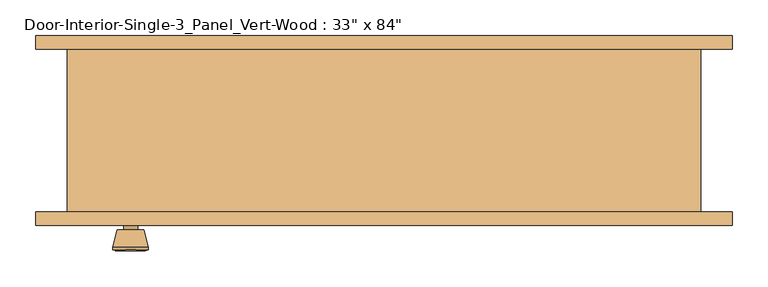
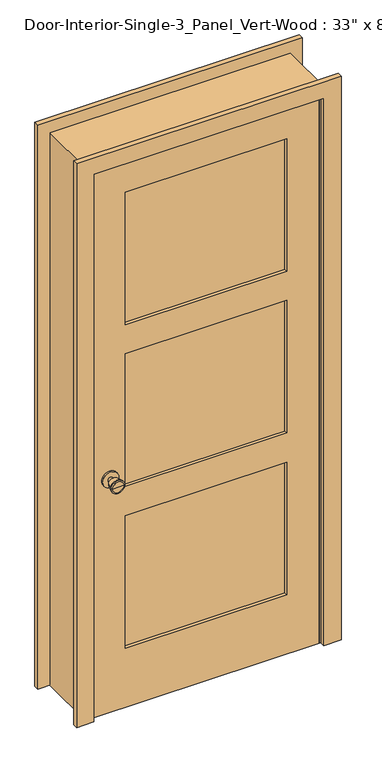
"""IFC4 building model written with IfcOpenShell, lengths in millimetres: door geometry."""

from ifc_helpers import new_model, si_unit, point, frame, frame_2d, origin, place, context, project, spatial, polyline, circle_curve, trimmed, segment, composite_curve, outline, extrude, faceted_brep, source, transform, mapped, element, save
from ifc_brep_helpers import plane_surface, cylinder_surface, revolved_surface, advanced_brep


def door_5abea521(model_context):
    return source(origin(), model_context, "Body", "SolidModel", [
        advanced_brep(
        [(-355.6, -70.2, 914.4), (-365.6, -70.2, 914.4), (-345.6, -70.2, 914.4), (-335.1241324, -21.2, 914.4), (-376.0758676, -21.2, 914.4), (-355.6, -21.2, 914.4), (-330.6, -23.0278681, 914.4), (-380.6, -23.0278681, 914.4), (-330.6, -26.4915463, 914.4), (-380.6, -26.4915463, 914.4), (-336.963764, -51.2, 914.4), (-374.236236, -51.2, 914.4), (-345.6, -51.2, 914.4), (-365.6, -51.2, 914.4)],
        [
            (0, 1),
            (1, 2, circle_curve(frame((-355.6, -70.2, 914.4), z_axis=(0.0, -1.0, 0.0), x_axis=(-1.0, 0.0, 0.0)), 10.0)),
            (2, 0),
            (2, 1, circle_curve(frame((-355.6, -70.2, 914.4), z_axis=(0.0, -1.0, 0.0), x_axis=(-1.0, 0.0, 0.0)), 10.0)),
            (3, 4, circle_curve(frame((-355.6, -21.2, 914.4), z_axis=(0.0, 1.0, 0.0), x_axis=(-1.0, 0.0, 0.0)), 20.4758676)),
            (4, 5),
            (5, 3),
            (4, 3, circle_curve(frame((-355.6, -21.2, 914.4), z_axis=(0.0, 1.0, 0.0), x_axis=(-1.0, 0.0, 0.0)), 20.4758676)),
            (6, 7, circle_curve(frame((-355.6, -23.0278681, 914.4), z_axis=(0.0, 1.0, 0.0), x_axis=(-1.0, 0.0, 0.0)), 25.0)),
            (7, 4),
            (3, 6),
            (7, 6, circle_curve(frame((-355.6, -23.0278681, 914.4), z_axis=(0.0, 1.0, 0.0), x_axis=(-1.0, 0.0, 0.0)), 25.0)),
            (8, 9, circle_curve(frame((-355.6, -26.4915463, 914.4), z_axis=(0.0, 1.0, 0.0), x_axis=(-1.0, 0.0, 0.0)), 25.0)),
            (9, 7),
            (6, 8),
            (9, 8, circle_curve(frame((-355.6, -26.4915463, 914.4), z_axis=(0.0, 1.0, 0.0), x_axis=(-1.0, 0.0, 0.0)), 25.0)),
            (10, 11, circle_curve(frame((-355.6, -51.2, 914.4), z_axis=(0.0, 1.0, 0.0), x_axis=(-1.0, 0.0, 0.0)), 18.636236)),
            (11, 9),
            (8, 10),
            (11, 10, circle_curve(frame((-355.6, -51.2, 914.4), z_axis=(0.0, 1.0, 0.0), x_axis=(-1.0, 0.0, 0.0)), 18.636236)),
            (12, 13, circle_curve(frame((-355.6, -51.2, 914.4), z_axis=(0.0, 1.0, 0.0), x_axis=(-1.0, 0.0, 0.0)), 10.0)),
            (13, 11),
            (10, 12),
            (13, 12, circle_curve(frame((-355.6, -51.2, 914.4), z_axis=(0.0, 1.0, 0.0), x_axis=(-1.0, 0.0, 0.0)), 10.0)),
            (1, 13),
            (12, 2),
        ],
        [
            plane_surface(frame((-355.6, -70.2, 914.4), z_axis=(0.0, -1.0, 0.0), x_axis=(-1.0, 0.0, 0.0))),
            plane_surface(frame((-355.6, -21.2, 914.4), z_axis=(0.0, 1.0, 0.0), x_axis=(-1.0, 0.0, 0.0))),
            revolved_surface(polyline([(-376.0758676, -21.2, 914.4), (-380.6, -23.0278681, 914.4)]), (-355.6, -70.2, 914.4), (0.0, -1.0, 0.0)),
            cylinder_surface(frame((-355.6, -70.2, 914.4), z_axis=(0.0, -1.0, 0.0), x_axis=(-1.0, 0.0, 0.0)), 25.0),
            revolved_surface(polyline([(-380.6, -26.4915463, 914.4), (-374.236236, -51.2, 914.4)]), (-355.6, -70.2, 914.4), (0.0, -1.0, 0.0)),
            plane_surface(frame((-355.6, -51.2, 914.4), z_axis=(0.0, -1.0, 0.0), x_axis=(-1.0, 0.0, 0.0))),
            cylinder_surface(frame((-355.6, -70.2, 914.4), z_axis=(0.0, -1.0, 0.0), x_axis=(-1.0, 0.0, 0.0)), 10.0),
        ],
        [
            (0, [[1, 2, 3]]),
            (0, [[-3, 4, -1]]),
            (1, [[5, 6, 7]]),
            (1, [[8, -7, -6]]),
            (2, [[9, 10, -5, 11]]),
            (2, [[12, -11, -8, -10]]),
            (3, [[13, 14, -9, 15]]),
            (3, [[16, -15, -12, -14]]),
            (4, [[17, 18, -13, 19]]),
            (4, [[20, -19, -16, -18]]),
            (5, [[21, 22, -17, 23]]),
            (5, [[24, -23, -20, -22]]),
            (6, [[-2, 25, -21, 26]]),
            (6, [[-4, -26, -24, -25]]),
        ],
    ),
        extrude(outline(composite_curve([segment(trimmed(circle_curve(frame_2d((914.4, -355.6)), 30.0), [point((914.4, -385.6))], [point((914.4, -325.6))], False, "CARTESIAN"), True, "CONTINUOUS"), segment(trimmed(circle_curve(frame_2d((914.4, -355.6)), 30.0), [point((914.4, -325.6))], [point((914.4, -385.6))], False, "CARTESIAN"), True, "CONTINUOUS")], self_intersect=False)), frame((0.0, -76.2, 0.0), z_axis=(0.0, 1.0, 0.0), x_axis=(0.0, 0.0, 1.0)), (0.0, 0.0, 1.0), 6.0),
        advanced_brep(
        [(-355.6, -117.125, 914.4), (-345.6, -117.125, 914.4), (-365.6, -117.125, 914.4), (-335.1241324, -166.125, 914.4), (-355.6, -166.125, 914.4), (-376.0758676, -166.125, 914.4), (-330.6, -164.2971319, 914.4), (-380.6, -164.2971319, 914.4), (-330.6, -160.8334537, 914.4), (-380.6, -160.8334537, 914.4), (-336.963764, -136.125, 914.4), (-374.236236, -136.125, 914.4), (-345.6, -136.125, 914.4), (-365.6, -136.125, 914.4)],
        [
            (0, 1),
            (1, 2, circle_curve(frame((-355.6, -117.125, 914.4), z_axis=(0.0, 1.0, 0.0), x_axis=(-1.0, 0.0, 0.0)), 10.0)),
            (2, 0),
            (2, 1, circle_curve(frame((-355.6, -117.125, 914.4), z_axis=(0.0, 1.0, 0.0), x_axis=(-1.0, 0.0, 0.0)), 10.0)),
            (3, 4),
            (4, 5),
            (5, 3, circle_curve(frame((-355.6, -166.125, 914.4), z_axis=(0.0, -1.0, 0.0), x_axis=(-1.0, 0.0, 0.0)), 20.4758676)),
            (3, 5, circle_curve(frame((-355.6, -166.125, 914.4), z_axis=(0.0, -1.0, 0.0), x_axis=(-1.0, 0.0, 0.0)), 20.4758676)),
            (6, 3),
            (5, 7),
            (7, 6, circle_curve(frame((-355.6, -164.2971319, 914.4), z_axis=(0.0, -1.0, 0.0), x_axis=(-1.0, 0.0, 0.0)), 25.0)),
            (6, 7, circle_curve(frame((-355.6, -164.2971319, 914.4), z_axis=(0.0, -1.0, 0.0), x_axis=(-1.0, 0.0, 0.0)), 25.0)),
            (8, 6),
            (7, 9),
            (9, 8, circle_curve(frame((-355.6, -160.8334537, 914.4), z_axis=(0.0, -1.0, 0.0), x_axis=(-1.0, 0.0, 0.0)), 25.0)),
            (8, 9, circle_curve(frame((-355.6, -160.8334537, 914.4), z_axis=(0.0, -1.0, 0.0), x_axis=(-1.0, 0.0, 0.0)), 25.0)),
            (10, 8),
            (9, 11),
            (11, 10, circle_curve(frame((-355.6, -136.125, 914.4), z_axis=(0.0, -1.0, 0.0), x_axis=(-1.0, 0.0, 0.0)), 18.636236)),
            (10, 11, circle_curve(frame((-355.6, -136.125, 914.4), z_axis=(0.0, -1.0, 0.0), x_axis=(-1.0, 0.0, 0.0)), 18.636236)),
            (12, 10),
            (11, 13),
            (13, 12, circle_curve(frame((-355.6, -136.125, 914.4), z_axis=(0.0, -1.0, 0.0), x_axis=(-1.0, 0.0, 0.0)), 10.0)),
            (12, 13, circle_curve(frame((-355.6, -136.125, 914.4), z_axis=(0.0, -1.0, 0.0), x_axis=(-1.0, 0.0, 0.0)), 10.0)),
            (1, 12),
            (13, 2),
        ],
        [
            plane_surface(frame((-355.6, -117.125, 914.4), z_axis=(0.0, 1.0, 0.0), x_axis=(-1.0, 0.0, 0.0))),
            plane_surface(frame((-355.6, -166.125, 914.4), z_axis=(0.0, -1.0, 0.0), x_axis=(-1.0, 0.0, 0.0))),
            revolved_surface(polyline([(-376.0758676, -166.125, 914.4), (-380.6, -164.2971319, 914.4)]), (-355.6, -117.125, 914.4), (0.0, 1.0, 0.0)),
            cylinder_surface(frame((-355.6, -117.125, 914.4), z_axis=(0.0, 1.0, 0.0), x_axis=(-1.0, 0.0, 0.0)), 25.0),
            revolved_surface(polyline([(-380.6, -160.8334537, 914.4), (-374.236236, -136.125, 914.4)]), (-355.6, -117.125, 914.4), (0.0, 1.0, 0.0)),
            plane_surface(frame((-355.6, -136.125, 914.4), z_axis=(0.0, 1.0, 0.0), x_axis=(-1.0, 0.0, 0.0))),
            cylinder_surface(frame((-355.6, -117.125, 914.4), z_axis=(0.0, 1.0, 0.0), x_axis=(-1.0, 0.0, 0.0)), 10.0),
        ],
        [
            (0, [[1, 2, 3]]),
            (0, [[-3, 4, -1]]),
            (1, [[5, 6, 7]]),
            (1, [[-6, -5, 8]]),
            (2, [[9, -7, 10, 11]]),
            (2, [[-10, -8, -9, 12]]),
            (3, [[13, -11, 14, 15]]),
            (3, [[-14, -12, -13, 16]]),
            (4, [[17, -15, 18, 19]]),
            (4, [[-18, -16, -17, 20]]),
            (5, [[21, -19, 22, 23]]),
            (5, [[-22, -20, -21, 24]]),
            (6, [[25, -23, 26, -2]]),
            (6, [[-26, -24, -25, -4]]),
        ],
    ),
        extrude(outline(composite_curve([segment(trimmed(circle_curve(frame_2d((914.4, -355.6)), 30.0), [point((914.4, -385.6))], [point((914.4, -325.6))], False, "CARTESIAN"), True, "CONTINUOUS"), segment(trimmed(circle_curve(frame_2d((914.4, -355.6)), 30.0), [point((914.4, -325.6))], [point((914.4, -385.6))], False, "CARTESIAN"), True, "CONTINUOUS")], self_intersect=False)), frame((0.0, -117.125, 0.0), z_axis=(0.0, 1.0, 0.0), x_axis=(0.0, 0.0, 1.0)), (0.0, 0.0, 1.0), 6.0),
        faceted_brep([(444.5, -111.125, 0.0), (419.1, -111.125, 0.0), (419.1, -76.2, 0.0), (406.4, -76.2, 0.0), (406.4, -41.275, 0.0), (419.1, -41.275, 0.0), (419.1, 117.475, 0.0), (444.5, 117.475, 0.0), (444.5, 117.475, 2159.0), (444.5, -111.125, 2159.0), (419.1, 117.475, 2133.6), (-419.1, 117.475, 2133.6), (-419.1, 117.475, 0.0), (-444.5, 117.475, 0.0), (-444.5, 117.475, 2159.0), (419.1, -41.275, 2133.6), (406.4, -41.275, 2120.9), (-406.4, -41.275, 2120.9), (-406.4, -41.275, 0.0), (-419.1, -41.275, 0.0), (-419.1, -41.275, 2133.6), (406.4, -76.2, 2120.9), (419.1, -76.2, 2133.6), (-419.1, -76.2, 2133.6), (-419.1, -76.2, 0.0), (-406.4, -76.2, 0.0), (-406.4, -76.2, 2120.9), (419.1, -111.125, 2133.6), (-444.5, -111.125, 2159.0), (-444.5, -111.125, 0.0), (-419.1, -111.125, 0.0), (-419.1, -111.125, 2133.6)], [[[0, 1, 2, 3, 4, 5, 6, 7]], [[7, 8, 9, 0]], [[6, 10, 11, 12, 13, 14, 8, 7]], [[5, 15, 10, 6]], [[4, 16, 17, 18, 19, 20, 15, 5]], [[3, 21, 16, 4]], [[2, 22, 23, 24, 25, 26, 21, 3]], [[1, 27, 22, 2]], [[0, 9, 28, 29, 30, 31, 27, 1]], [[8, 14, 28, 9]], [[15, 20, 11, 10]], [[21, 26, 17, 16]], [[27, 31, 23, 22]], [[29, 13, 12, 19, 18, 25, 24, 30]], [[14, 13, 29, 28]], [[20, 19, 12, 11]], [[26, 25, 18, 17]], [[31, 30, 24, 23]]]),
        extrude(outline(polyline([(2133.6, -419.1), (0.0, -419.1), (0.0, 419.1), (2133.6, 419.1), (2133.6, -419.1)]), holes=[polyline([(2014.5375, -298.45), (2014.5375, 298.45), (1496.4833333, 298.45), (1496.4833333, -298.45), (2014.5375, -298.45)]), polyline([(749.8291667, -298.45), (749.8291667, 298.45), (231.775, 298.45), (231.775, -298.45), (749.8291667, -298.45)]), polyline([(1382.1833333, -298.45), (1382.1833333, 298.45), (864.1291667, 298.45), (864.1291667, -298.45), (1382.1833333, -298.45)])]), frame((0.0, -111.125, 0.0), z_axis=(0.0, 1.0, 0.0), x_axis=(0.0, 0.0, 1.0)), (0.0, 0.0, 1.0), 34.925),
        extrude(outline(polyline([(298.45, -87.8416667), (298.45, -99.4833333), (-298.45, -99.4833333), (-298.45, -87.8416667), (298.45, -87.8416667)])), frame((0.0, 0.0, 1496.4833333), z_axis=(0.0, 0.0, 1.0), x_axis=(1.0, 0.0, 0.0)), (0.0, 0.0, 1.0), 518.0541667),
        extrude(outline(polyline([(298.45, -87.8416667), (298.45, -99.4833333), (-298.45, -99.4833333), (-298.45, -87.8416667), (298.45, -87.8416667)])), frame((0.0, 0.0, 231.775), z_axis=(0.0, 0.0, 1.0), x_axis=(1.0, 0.0, 0.0)), (0.0, 0.0, 1.0), 518.0541667),
        extrude(outline(polyline([(298.45, -87.8416667), (298.45, -99.4833333), (-298.45, -99.4833333), (-298.45, -87.8416667), (298.45, -87.8416667)])), frame((0.0, 0.0, 864.1291667), z_axis=(0.0, 0.0, 1.0), x_axis=(1.0, 0.0, 0.0)), (0.0, 0.0, 1.0), 518.0541667),
        extrude(outline(polyline([(0.0, 488.95), (2203.45, 488.95), (2203.45, -488.95), (0.0, -488.95), (0.0, -425.45), (2139.95, -425.45), (2139.95, 425.45), (0.0, 425.45), (0.0, 488.95)])), frame((0.0, -130.175, 0.0), z_axis=(0.0, 1.0, 0.0), x_axis=(0.0, 0.0, 1.0)), (0.0, 0.0, 1.0), 19.05),
        extrude(outline(polyline([(0.0, 488.95), (2203.45, 488.95), (2203.45, -488.95), (0.0, -488.95), (0.0, -425.45), (2139.95, -425.45), (2139.95, 425.45), (0.0, 425.45), (0.0, 488.95)])), frame((0.0, 117.475, 0.0), z_axis=(0.0, 1.0, 0.0), x_axis=(0.0, 0.0, 1.0)), (0.0, 0.0, 1.0), 19.05),
    ])


if __name__ == "__main__":
    model = new_model("IFC4")
    model_context = context("Model", 3, world=origin())
    ifc_project = project(units=[si_unit("LENGTHUNIT", "METRE", prefix="MILLI")], contexts=[model_context])
    site = spatial("IfcSite", under=ifc_project)
    building = spatial("IfcBuilding", under=site)
    placement = place(None, origin())
    door_shape = door_5abea521(model_context)
    element("IfcDoor", 1, ObjectType="Door-Interior-Single-3_Panel_Vert-Wood : 33\" x 84\"", at=placement, inside=building, context=model_context, shape_type="MappedRepresentation", body=[
        mapped(door_shape, transform((0.0, 0.0, 0.0), x_axis=(1.0, 0.0, 0.0), y_axis=(0.0, 1.0, 0.0), z_axis=(0.0, 0.0, 1.0))),
    ])
    save(model, "model.ifc")

# Revit data of these elements
# Type "Door-Interior-Single-3_Panel_Vert-Wood : 33\" x 84\""
#   Type Mark = "11"
#   Assembly Code = "C1020300"
#   Analytic Construction = "Wooden"
#   Top Rail = 0' - 4 11/16"
#   Thickness = 0' - 1 3/8"
#   Thermal Resistance (R) = 2.5876 (h·ft²·°F)/BTU
#   Swing Angle [instance default] = 90.00°
#   Stiles = 0' - 4 3/4"
#   Rough Width = 2' - 11"
#   Rough Height = 7' - 1"
#   Intermediate Rail = 0' - 4 1/2"
#   Height = 7' - 0"
#   Width = 2' - 9"
#   Heat Transfer Coefficient (U) = 0.3865 BTU/(h·ft²·°F)
#   Bottom Rail = 0' - 9 1/8"
#   Trim Material = Cherry
#   Panel Material = Cherry
#   Frame Material = Cherry
#   Door Handle Material = Aluminum
#   Visual Light Transmittance = 0
#   Solar Heat Gain Coefficient = 0
#   Wall Closure = (empty or 0)
#   Function = (empty or 0)
# Element 1 (IfcDoor, "Door-Interior-Single-3_Panel_Vert-Wood : 33\" x 84\"")
#   Materials on its faces: "Cherry", "Aluminum"
# Materials
#   "Cherry": class "Wood", colour RGB 226 177 128, transparency 0, Description = "Prunus Serotina", Cost = 0
#   "Aluminum": class "Metal", colour RGB 247 247 247, transparency 0, Description = "Aluminum 6061", Cost = 0
